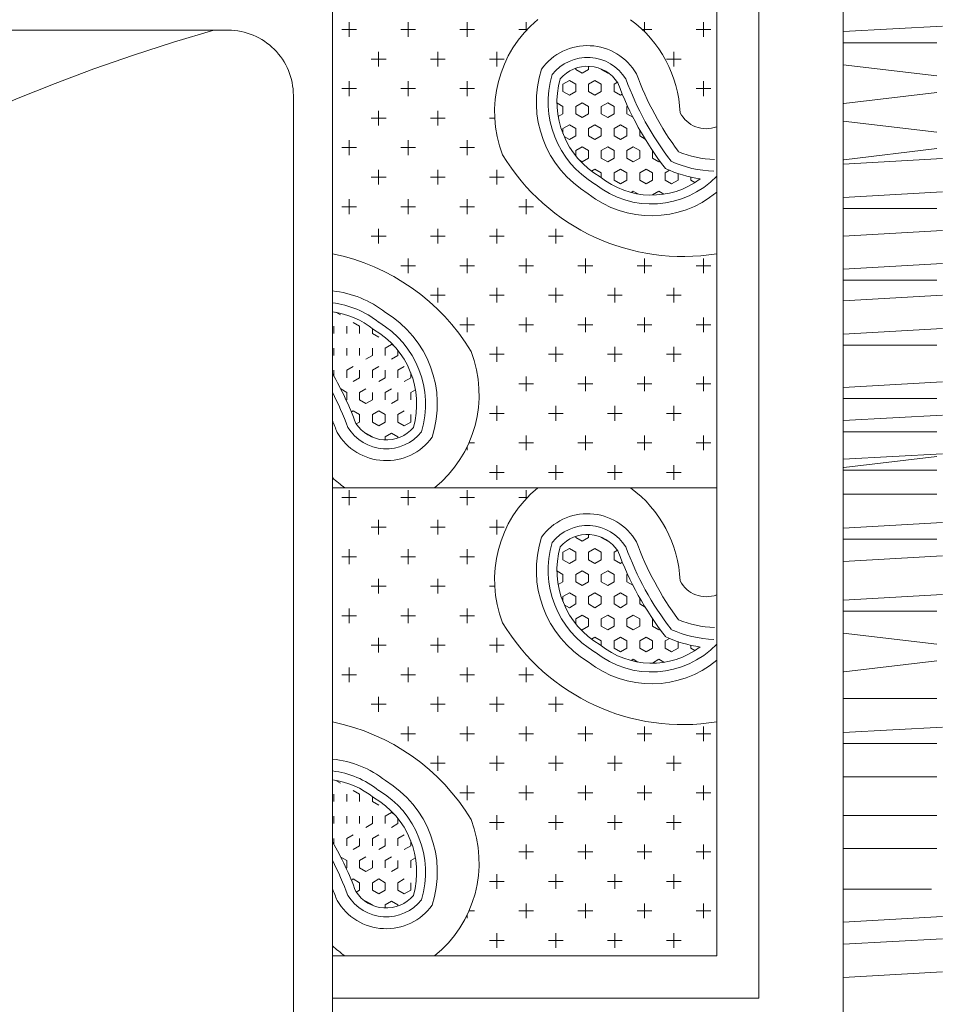
# Model space of a CAD drawing. Units: inches. Extents: x -638 to 186, y -762 to 59.
# Tile 9 of 31: x -117.58 to -100.41, y -492.33 to -474.18. Entities that reach past the tile are written whole.
import ezdxf

# ---------------------------------------------------------------- set-up
doc = ezdxf.new("R2010")
doc.units = ezdxf.units.IN
doc.layers.add('A-ANNO-DIMS', color=2, linetype='Continuous', lineweight=18)
doc.layers.add('furn', color=8, linetype='Continuous', lineweight=13)
doc.styles.get("Standard").update_dxf_attribs({"font": 'arial.ttf'})
doc.dimstyles.new('ISO-25', dxfattribs={"dimtxt": 4, "dimasz": 4, "dimexe": 1.25, "dimexo": 0.625, "dimtad": 0, "dimlunit": 4, "dimtxsty": 'Standard', "dimcen": 2.5, "dimclrt": 256, "dimadec": 0, "dimazin": 0, "dimtfac": 1, "dimtmove": 0, "dimatfit": 3, "dimfxl": 1, "dimfxlon": 1, "dimarcsym": 0})

# ---------------------------------------------------------------- blocks, each defined once
blk = doc.blocks.new('BED-DOUBLE-WITH-NIGHTSTANDS')
for p, q in [((57.828, 13.164), (57.828, 58.468)), ((22.077, 11.964), (56.628, 11.964)), ((20.158, 11.244), (58.548, 11.244)), ((39.99, 3.384), (39.99, 11.244)), ((40.767, 4.161), (40.767, 11.244)), ((42.588, 11.09), (42.524, 10.979)), ((42.932, 11.215), (42.819, 11.215)), ((43.34, 11.215), (43.204, 11.215)), ((43.748, 11.215), (43.612, 11.215)), ((44.002, 11.184), (43.952, 11.097)), ((45.948, 10.8), (45.948, 11.072)), ((47.036, 10.8), (47.036, 11.072)), ((48.125, 10.8), (48.125, 11.072)), ((49.213, 10.8), (49.213, 11.072)), ((49.395, 11.244), (49.395, 4.161)), ((51.216, 11.09), (51.151, 10.979)), ((51.56, 11.215), (51.447, 11.215)), ((51.968, 11.215), (51.832, 11.215)), ((52.376, 11.215), (52.24, 11.215)), ((52.63, 11.184), (52.58, 11.097)), ((54.576, 10.8), (54.576, 11.072)), ((55.664, 10.8), (55.664, 11.072)), ((56.752, 10.8), (56.752, 11.072)), ((57.841, 10.8), (57.841, 11.072)), ((42.164, 10.895), (42.184, 10.861)), ((42.381, 10.99), (42.388, 10.979)), ((42.524, 10.979), (42.388, 10.979)), ((42.932, 10.979), (42.796, 10.979)), ((42.932, 10.979), (43, 10.861)), ((43.34, 10.979), (43.204, 10.979)), ((43.748, 10.979), (43.612, 10.979)), ((45.812, 10.936), (46.084, 10.936)), ((46.9, 10.936), (47.172, 10.936)), ((47.989, 10.936), (48.261, 10.936)), ((49.077, 10.936), (49.349, 10.936)), ((50.792, 10.895), (50.811, 10.861)), ((51.009, 10.99), (51.015, 10.979)), ((51.151, 10.979), (51.015, 10.979)), ((51.56, 10.979), (51.424, 10.979)), ((51.56, 10.979), (51.628, 10.861)), ((51.968, 10.979), (51.832, 10.979)), ((52.376, 10.979), (52.24, 10.979)), ((54.44, 10.936), (54.712, 10.936)), ((55.528, 10.936), (55.8, 10.936)), ((56.616, 10.936), (56.888, 10.936)), ((57.705, 10.936), (57.977, 10.936)), ((41.943, 10.806), (41.98, 10.743)), ((42.116, 10.743), (41.98, 10.743)), ((42.184, 10.861), (42.116, 10.743)), ((42.388, 10.743), (42.32, 10.625)), ((42.524, 10.743), (42.388, 10.743)), ((42.524, 10.743), (42.592, 10.625)), ((42.728, 10.861), (42.796, 10.743)), ((42.932, 10.743), (42.796, 10.743)), ((43.34, 10.743), (43.204, 10.743)), ((43.748, 10.743), (43.612, 10.743)), ((43.816, 10.861), (43.748, 10.743)), ((50.571, 10.806), (50.607, 10.743)), ((50.743, 10.743), (50.607, 10.743)), ((50.811, 10.861), (50.743, 10.743)), ((51.015, 10.743), (50.947, 10.625)), ((51.151, 10.743), (51.015, 10.743)), ((51.151, 10.743), (51.219, 10.625)), ((51.355, 10.861), (51.424, 10.743)), ((51.56, 10.743), (51.424, 10.743)), ((51.968, 10.743), (51.832, 10.743)), ((52.376, 10.743), (52.24, 10.743)), ((52.444, 10.861), (52.376, 10.743)), ((41.776, 10.625), (41.708, 10.508)), ((41.77, 10.636), (41.776, 10.625)), ((42.32, 10.625), (42.388, 10.508)), ((43.136, 10.625), (43.204, 10.508)), ((45.404, 10.256), (45.404, 10.528)), ((46.492, 10.256), (46.492, 10.528)), ((47.581, 10.256), (47.581, 10.528)), ((48.669, 10.256), (48.669, 10.528)), ((50.403, 10.625), (50.335, 10.508)), ((50.397, 10.636), (50.403, 10.625)), ((50.947, 10.625), (51.015, 10.508)), ((51.764, 10.625), (51.832, 10.508)), ((54.032, 10.256), (54.032, 10.528)), ((55.12, 10.256), (55.12, 10.528)), ((56.208, 10.256), (56.208, 10.528)), ((57.297, 10.256), (57.297, 10.528)), ((41.708, 10.508), (41.699, 10.508)), ((41.98, 10.508), (41.912, 10.39)), ((41.912, 10.39), (41.98, 10.272)), ((42.116, 10.508), (41.98, 10.508)), ((42.116, 10.508), (42.184, 10.39)), ((42.184, 10.39), (42.116, 10.272)), ((42.524, 10.508), (42.388, 10.508)), ((42.728, 10.39), (42.796, 10.272)), ((42.932, 10.508), (42.796, 10.508)), ((42.932, 10.508), (43, 10.39)), ((43.34, 10.508), (43.204, 10.508)), ((43.612, 10.508), (43.544, 10.39)), ((43.703, 10.508), (43.612, 10.508)), ((45.268, 10.392), (45.54, 10.392)), ((46.356, 10.392), (46.628, 10.392)), ((47.445, 10.392), (47.717, 10.392)), ((48.533, 10.392), (48.805, 10.392)), ((50.335, 10.508), (50.327, 10.508)), ((50.607, 10.508), (50.539, 10.39)), ((50.539, 10.39), (50.607, 10.272)), ((50.743, 10.508), (50.607, 10.508)), ((50.743, 10.508), (50.811, 10.39)), ((50.811, 10.39), (50.743, 10.272)), ((51.151, 10.508), (51.015, 10.508)), ((51.355, 10.39), (51.424, 10.272)), ((51.56, 10.508), (51.424, 10.508)), ((51.56, 10.508), (51.628, 10.39)), ((51.968, 10.508), (51.832, 10.508)), ((52.24, 10.508), (52.172, 10.39)), ((52.33, 10.508), (52.24, 10.508)), ((53.896, 10.392), (54.168, 10.392)), ((54.984, 10.392), (55.256, 10.392)), ((56.072, 10.392), (56.344, 10.392)), ((57.161, 10.392), (57.433, 10.392)), ((41.708, 10.272), (41.649, 10.272)), ((41.708, 10.272), (41.776, 10.154)), ((42.116, 10.272), (41.98, 10.272)), ((42.524, 10.272), (42.388, 10.272)), ((42.524, 10.272), (42.592, 10.154)), ((42.932, 10.272), (42.796, 10.272)), ((43.34, 10.272), (43.204, 10.272)), ((43.34, 10.272), (43.408, 10.154)), ((50.335, 10.272), (50.277, 10.272)), ((50.335, 10.272), (50.403, 10.154)), ((50.743, 10.272), (50.607, 10.272)), ((51.151, 10.272), (51.015, 10.272)), ((51.151, 10.272), (51.219, 10.154)), ((51.56, 10.272), (51.424, 10.272)), ((51.968, 10.272), (51.832, 10.272)), ((51.968, 10.272), (52.036, 10.154)), ((41.708, 10.036), (41.685, 10.036)), ((41.776, 10.154), (41.708, 10.036)), ((41.98, 10.036), (41.912, 9.919)), ((42.116, 10.036), (41.98, 10.036)), ((42.116, 10.036), (42.184, 9.919)), ((42.32, 10.154), (42.388, 10.036)), ((42.524, 10.036), (42.388, 10.036)), ((42.932, 10.036), (42.796, 10.036)), ((42.932, 10.036), (43, 9.919)), ((43.136, 10.154), (43.204, 10.036)), ((43.297, 10.036), (43.204, 10.036)), ((43.408, 10.154), (43.381, 10.108)), ((44.86, 9.711), (44.86, 9.983)), ((45.948, 9.711), (45.948, 9.983)), ((47.036, 9.711), (47.036, 9.983)), ((48.125, 9.711), (48.125, 9.983)), ((49.213, 9.711), (49.213, 9.983)), ((50.335, 10.036), (50.313, 10.036)), ((50.403, 10.154), (50.335, 10.036)), ((50.607, 10.036), (50.539, 9.919)), ((50.743, 10.036), (50.607, 10.036)), ((50.743, 10.036), (50.811, 9.919)), ((50.947, 10.154), (51.015, 10.036)), ((51.151, 10.036), (51.015, 10.036)), ((51.56, 10.036), (51.424, 10.036)), ((51.56, 10.036), (51.628, 9.919)), ((51.764, 10.154), (51.832, 10.036)), ((51.925, 10.036), (51.832, 10.036)), ((52.036, 10.154), (52.009, 10.108)), ((53.487, 9.711), (53.487, 9.983)), ((54.576, 9.711), (54.576, 9.983)), ((55.664, 9.711), (55.664, 9.983)), ((56.752, 9.711), (56.752, 9.983)), ((57.841, 9.711), (57.841, 9.983)), ((41.912, 9.919), (41.98, 9.801)), ((42.116, 9.801), (41.98, 9.801)), ((42.524, 9.801), (42.388, 9.801)), ((42.524, 9.801), (42.574, 9.713)), ((42.728, 9.919), (42.796, 9.801)), ((42.888, 9.801), (42.796, 9.801)), ((44.724, 9.847), (44.996, 9.847)), ((45.812, 9.847), (46.084, 9.847)), ((46.9, 9.847), (47.172, 9.847)), ((47.989, 9.847), (48.261, 9.847)), ((49.077, 9.847), (49.349, 9.847)), ((50.539, 9.919), (50.607, 9.801)), ((50.743, 9.801), (50.607, 9.801)), ((51.151, 9.801), (51.015, 9.801)), ((51.151, 9.801), (51.202, 9.713)), ((51.355, 9.919), (51.424, 9.801)), ((51.516, 9.801), (51.424, 9.801)), ((53.351, 9.847), (53.623, 9.847)), ((54.44, 9.847), (54.712, 9.847)), ((55.528, 9.847), (55.8, 9.847)), ((56.616, 9.847), (56.888, 9.847)), ((57.705, 9.847), (57.977, 9.847)), ((44.316, 9.167), (44.316, 9.439)), ((45.404, 9.167), (45.404, 9.439)), ((46.492, 9.167), (46.492, 9.439)), ((47.581, 9.167), (47.581, 9.439)), ((48.669, 9.167), (48.669, 9.439)), ((52.943, 9.167), (52.943, 9.439)), ((54.032, 9.167), (54.032, 9.439)), ((55.12, 9.167), (55.12, 9.439)), ((56.208, 9.167), (56.208, 9.439)), ((57.297, 9.167), (57.297, 9.439)), ((44.18, 9.303), (44.452, 9.303)), ((45.268, 9.303), (45.54, 9.303)), ((46.356, 9.303), (46.628, 9.303)), ((47.445, 9.303), (47.717, 9.303)), ((48.533, 9.303), (48.805, 9.303)), ((52.807, 9.303), (53.079, 9.303)), ((53.896, 9.303), (54.168, 9.303)), ((54.984, 9.303), (55.256, 9.303)), ((56.072, 9.303), (56.344, 9.303)), ((57.161, 9.303), (57.433, 9.303)), ((43.771, 8.623), (43.771, 8.895)), ((44.86, 8.623), (44.86, 8.895)), ((45.948, 8.623), (45.948, 8.895)), ((47.036, 8.623), (47.036, 8.895)), ((48.125, 8.623), (48.125, 8.895)), ((49.213, 8.623), (49.213, 8.895)), ((52.399, 8.623), (52.399, 8.895)), ((53.487, 8.623), (53.487, 8.895)), ((54.576, 8.623), (54.576, 8.895)), ((55.664, 8.623), (55.664, 8.895)), ((56.752, 8.623), (56.752, 8.895)), ((57.841, 8.623), (57.841, 8.895)), ((41.459, 8.759), (41.528, 8.759)), ((41.595, 8.623), (41.595, 8.728)), ((43.635, 8.759), (43.907, 8.759)), ((44.724, 8.759), (44.996, 8.759)), ((45.812, 8.759), (46.084, 8.759)), ((46.9, 8.759), (47.172, 8.759)), ((47.989, 8.759), (48.261, 8.759)), ((49.077, 8.759), (49.349, 8.759)), ((50.086, 8.759), (50.155, 8.759)), ((50.222, 8.623), (50.222, 8.728)), ((52.263, 8.759), (52.535, 8.759)), ((53.351, 8.759), (53.623, 8.759)), ((54.44, 8.759), (54.712, 8.759)), ((55.528, 8.759), (55.8, 8.759)), ((56.616, 8.759), (56.888, 8.759)), ((57.705, 8.759), (57.977, 8.759)), ((41.051, 8.079), (41.051, 8.351)), ((42.139, 8.079), (42.139, 8.351)), ((43.227, 8.079), (43.227, 8.351)), ((44.316, 8.079), (44.316, 8.351)), ((45.404, 8.079), (45.404, 8.351)), ((46.492, 8.079), (46.492, 8.351)), ((47.581, 8.253), (47.581, 8.351)), ((48.669, 8.079), (48.669, 8.351)), ((49.678, 8.079), (49.678, 8.351)), ((50.767, 8.079), (50.767, 8.351)), ((51.855, 8.079), (51.855, 8.351)), ((52.943, 8.079), (52.943, 8.351)), ((54.032, 8.079), (54.032, 8.351)), ((55.12, 8.079), (55.12, 8.351)), ((56.208, 8.253), (56.208, 8.351)), ((57.297, 8.079), (57.297, 8.351)), ((40.914, 8.215), (41.187, 8.215)), ((42.003, 8.215), (42.275, 8.215)), ((43.091, 8.215), (43.363, 8.215)), ((44.18, 8.215), (44.452, 8.215)), ((45.268, 8.215), (45.54, 8.215)), ((46.356, 8.215), (46.628, 8.215)), ((48.533, 8.215), (48.805, 8.215)), ((49.542, 8.215), (49.814, 8.215)), ((50.63, 8.215), (50.903, 8.215)), ((51.719, 8.215), (51.991, 8.215)), ((52.807, 8.215), (53.079, 8.215)), ((53.896, 8.215), (54.168, 8.215)), ((54.984, 8.215), (55.256, 8.215)), ((57.161, 8.215), (57.433, 8.215)), ((41.595, 7.535), (41.595, 7.807)), ((42.683, 7.535), (42.683, 7.807)), ((43.771, 7.535), (43.771, 7.807)), ((44.86, 7.535), (44.86, 7.807)), ((45.948, 7.535), (45.948, 7.807)), ((49.213, 7.653), (49.213, 7.807)), ((50.222, 7.535), (50.222, 7.807)), ((51.311, 7.535), (51.311, 7.807)), ((52.399, 7.535), (52.399, 7.807)), ((53.487, 7.535), (53.487, 7.807)), ((54.576, 7.535), (54.576, 7.807)), ((57.841, 7.653), (57.841, 7.807)), ((41.459, 7.671), (41.731, 7.671)), ((42.547, 7.671), (42.819, 7.671)), ((43.635, 7.671), (43.907, 7.671)), ((44.724, 7.671), (44.996, 7.671)), ((45.812, 7.671), (46.084, 7.671)), ((49.195, 7.671), (49.349, 7.671)), ((50.086, 7.671), (50.358, 7.671)), ((51.175, 7.671), (51.447, 7.671)), ((52.263, 7.671), (52.535, 7.671)), ((53.351, 7.671), (53.623, 7.671)), ((54.44, 7.671), (54.712, 7.671)), ((57.822, 7.671), (57.977, 7.671)), ((41.051, 6.99), (41.051, 7.263)), ((42.139, 6.99), (42.139, 7.263)), ((43.227, 6.99), (43.227, 7.263)), ((44.316, 6.99), (44.316, 7.263)), ((45.404, 6.99), (45.404, 7.263)), ((49.678, 6.99), (49.678, 7.263)), ((50.767, 6.99), (50.767, 7.263)), ((51.855, 6.99), (51.855, 7.263)), ((52.943, 6.99), (52.943, 7.263)), ((54.032, 6.99), (54.032, 7.263)), ((40.914, 7.127), (41.187, 7.127)), ((42.003, 7.127), (42.275, 7.127)), ((43.091, 7.127), (43.363, 7.127)), ((44.18, 7.127), (44.452, 7.127)), ((45.268, 7.127), (45.54, 7.127)), ((47.661, 6.995), (47.611, 7.082)), ((47.797, 6.995), (47.861, 7.105)), ((49.542, 7.127), (49.814, 7.127)), ((50.63, 7.127), (50.903, 7.127)), ((51.719, 7.127), (51.991, 7.127)), ((52.807, 7.127), (53.079, 7.127)), ((53.896, 7.127), (54.168, 7.127)), ((56.289, 6.995), (56.238, 7.082)), ((56.425, 6.995), (56.488, 7.105)), ((47.185, 6.877), (47.239, 6.971)), ((47.297, 6.995), (47.389, 6.995)), ((47.457, 6.877), (47.389, 6.995)), ((47.661, 6.995), (47.797, 6.995)), ((48.001, 6.877), (48.069, 6.995)), ((48.069, 6.995), (48.205, 6.995)), ((48.273, 6.877), (48.205, 6.995)), ((55.813, 6.877), (55.867, 6.971)), ((55.924, 6.995), (56.017, 6.995)), ((56.085, 6.877), (56.017, 6.995)), ((56.289, 6.995), (56.425, 6.995)), ((56.629, 6.877), (56.697, 6.995)), ((56.697, 6.995), (56.833, 6.995)), ((56.901, 6.877), (56.833, 6.995)), ((41.595, 6.446), (41.595, 6.718)), ((42.683, 6.446), (42.683, 6.718)), ((43.771, 6.446), (43.771, 6.718)), ((44.86, 6.446), (44.86, 6.718)), ((46.888, 6.76), (46.981, 6.76)), ((47.049, 6.642), (46.981, 6.76)), ((47.253, 6.76), (47.185, 6.877)), ((47.253, 6.76), (47.389, 6.76)), ((47.389, 6.76), (47.457, 6.877)), ((47.593, 6.642), (47.661, 6.76)), ((47.661, 6.76), (47.797, 6.76)), ((47.865, 6.642), (47.797, 6.76)), ((48.069, 6.76), (48.001, 6.877)), ((48.069, 6.76), (48.205, 6.76)), ((48.205, 6.76), (48.273, 6.877)), ((48.409, 6.642), (48.477, 6.76)), ((48.477, 6.76), (48.5, 6.76)), ((50.222, 6.446), (50.222, 6.718)), ((51.311, 6.446), (51.311, 6.718)), ((52.399, 6.446), (52.399, 6.718)), ((53.487, 6.446), (53.487, 6.718)), ((55.515, 6.76), (55.609, 6.76)), ((55.677, 6.642), (55.609, 6.76)), ((55.881, 6.76), (55.813, 6.877)), ((55.881, 6.76), (56.017, 6.76)), ((56.017, 6.76), (56.085, 6.877)), ((56.221, 6.642), (56.289, 6.76)), ((56.289, 6.76), (56.425, 6.76)), ((56.493, 6.642), (56.425, 6.76)), ((56.697, 6.76), (56.629, 6.877)), ((56.697, 6.76), (56.833, 6.76)), ((56.833, 6.76), (56.901, 6.877)), ((57.037, 6.642), (57.105, 6.76)), ((57.105, 6.76), (57.128, 6.76)), ((41.459, 6.582), (41.731, 6.582)), ((42.547, 6.582), (42.819, 6.582)), ((43.635, 6.582), (43.907, 6.582)), ((44.724, 6.582), (44.996, 6.582)), ((46.777, 6.642), (46.803, 6.688)), ((46.845, 6.524), (46.777, 6.642)), ((46.981, 6.524), (47.049, 6.642)), ((47.661, 6.524), (47.593, 6.642)), ((47.797, 6.524), (47.865, 6.642)), ((48.477, 6.524), (48.409, 6.642)), ((50.086, 6.582), (50.358, 6.582)), ((51.175, 6.582), (51.447, 6.582)), ((52.263, 6.582), (52.535, 6.582)), ((53.351, 6.582), (53.623, 6.582)), ((55.405, 6.642), (55.431, 6.688)), ((55.473, 6.524), (55.405, 6.642)), ((55.609, 6.524), (55.677, 6.642)), ((56.289, 6.524), (56.221, 6.642)), ((56.425, 6.524), (56.493, 6.642)), ((57.105, 6.524), (57.037, 6.642)), ((46.573, 6.288), (46.641, 6.406)), ((46.641, 6.406), (46.605, 6.469)), ((46.845, 6.524), (46.981, 6.524)), ((47.185, 6.406), (47.253, 6.524)), ((47.253, 6.288), (47.185, 6.406)), ((47.253, 6.524), (47.389, 6.524)), ((47.457, 6.406), (47.389, 6.524)), ((47.389, 6.288), (47.457, 6.406)), ((47.661, 6.524), (47.797, 6.524)), ((48.001, 6.406), (48.069, 6.524)), ((48.069, 6.288), (48.001, 6.406)), ((48.069, 6.524), (48.205, 6.524)), ((48.273, 6.406), (48.205, 6.524)), ((48.205, 6.288), (48.273, 6.406)), ((48.477, 6.524), (48.536, 6.524)), ((55.201, 6.288), (55.269, 6.406)), ((55.269, 6.406), (55.232, 6.469)), ((55.473, 6.524), (55.609, 6.524)), ((55.813, 6.406), (55.881, 6.524)), ((55.881, 6.288), (55.813, 6.406)), ((55.881, 6.524), (56.017, 6.524)), ((56.085, 6.406), (56.017, 6.524)), ((56.017, 6.288), (56.085, 6.406)), ((56.289, 6.524), (56.425, 6.524)), ((56.629, 6.406), (56.697, 6.524)), ((56.697, 6.288), (56.629, 6.406)), ((56.697, 6.524), (56.833, 6.524)), ((56.901, 6.406), (56.833, 6.524)), ((56.833, 6.288), (56.901, 6.406)), ((57.105, 6.524), (57.164, 6.524)), ((41.051, 5.902), (41.051, 6.174)), ((42.139, 5.902), (42.139, 6.174)), ((43.227, 5.902), (43.227, 6.174)), ((44.316, 5.902), (44.316, 6.174)), ((46.482, 6.288), (46.573, 6.288)), ((46.777, 6.17), (46.845, 6.288)), ((46.845, 6.053), (46.777, 6.17)), ((46.845, 6.288), (46.981, 6.288)), ((47.049, 6.17), (46.981, 6.288)), ((46.981, 6.053), (47.049, 6.17)), ((47.253, 6.288), (47.389, 6.288)), ((47.593, 6.17), (47.661, 6.288)), ((47.661, 6.053), (47.593, 6.17)), ((47.661, 6.288), (47.797, 6.288)), ((47.865, 6.17), (47.797, 6.288)), ((47.797, 6.053), (47.865, 6.17)), ((48.069, 6.288), (48.205, 6.288)), ((48.409, 6.17), (48.477, 6.288)), ((48.415, 6.16), (48.409, 6.17)), ((48.477, 6.288), (48.486, 6.288)), ((49.678, 5.902), (49.678, 6.174)), ((50.767, 5.902), (50.767, 6.174)), ((51.855, 5.902), (51.855, 6.174)), ((52.943, 5.902), (52.943, 6.174)), ((55.11, 6.288), (55.201, 6.288)), ((55.405, 6.17), (55.473, 6.288)), ((55.473, 6.053), (55.405, 6.17)), ((55.473, 6.288), (55.609, 6.288)), ((55.677, 6.17), (55.609, 6.288)), ((55.609, 6.053), (55.677, 6.17)), ((55.881, 6.288), (56.017, 6.288)), ((56.221, 6.17), (56.289, 6.288)), ((56.289, 6.053), (56.221, 6.17)), ((56.289, 6.288), (56.425, 6.288)), ((56.493, 6.17), (56.425, 6.288)), ((56.425, 6.053), (56.493, 6.17)), ((56.697, 6.288), (56.833, 6.288)), ((57.037, 6.17), (57.105, 6.288)), ((57.043, 6.16), (57.037, 6.17)), ((57.105, 6.288), (57.113, 6.288)), ((40.914, 6.038), (41.187, 6.038)), ((42.003, 6.038), (42.275, 6.038)), ((43.091, 6.038), (43.363, 6.038)), ((44.18, 6.038), (44.452, 6.038)), ((46.369, 5.935), (46.437, 6.053)), ((46.437, 6.053), (46.573, 6.053)), ((46.641, 5.935), (46.573, 6.053)), ((46.845, 6.053), (46.981, 6.053)), ((47.185, 5.935), (47.253, 6.053)), ((47.253, 6.053), (47.389, 6.053)), ((47.457, 5.935), (47.389, 6.053)), ((47.661, 6.053), (47.797, 6.053)), ((48.001, 5.935), (48.069, 6.053)), ((48.069, 6.053), (48.205, 6.053)), ((48.242, 5.99), (48.205, 6.053)), ((49.542, 6.038), (49.814, 6.038)), ((50.63, 6.038), (50.903, 6.038)), ((51.719, 6.038), (51.991, 6.038)), ((52.807, 6.038), (53.079, 6.038)), ((54.996, 5.935), (55.064, 6.053)), ((55.064, 6.053), (55.201, 6.053)), ((55.269, 5.935), (55.201, 6.053)), ((55.473, 6.053), (55.609, 6.053)), ((55.813, 5.935), (55.881, 6.053)), ((55.881, 6.053), (56.017, 6.053)), ((56.085, 5.935), (56.017, 6.053)), ((56.289, 6.053), (56.425, 6.053)), ((56.629, 5.935), (56.697, 6.053)), ((56.697, 6.053), (56.833, 6.053)), ((56.869, 5.99), (56.833, 6.053)), ((46.437, 5.817), (46.369, 5.935)), ((46.437, 5.817), (46.573, 5.817)), ((46.573, 5.817), (46.641, 5.935)), ((46.777, 5.699), (46.845, 5.817)), ((46.845, 5.817), (46.981, 5.817)), ((47.049, 5.699), (46.981, 5.817)), ((47.253, 5.817), (47.185, 5.935)), ((47.253, 5.817), (47.389, 5.817)), ((47.389, 5.817), (47.457, 5.935)), ((47.597, 5.706), (47.661, 5.817)), ((47.661, 5.817), (47.797, 5.817)), ((47.804, 5.806), (47.797, 5.817)), ((48.021, 5.901), (48.001, 5.935)), ((55.064, 5.817), (54.996, 5.935)), ((55.064, 5.817), (55.201, 5.817)), ((55.201, 5.817), (55.269, 5.935)), ((55.405, 5.699), (55.473, 5.817)), ((55.473, 5.817), (55.609, 5.817)), ((55.677, 5.699), (55.609, 5.817)), ((55.881, 5.817), (55.813, 5.935)), ((55.881, 5.817), (56.017, 5.817)), ((56.017, 5.817), (56.085, 5.935)), ((56.225, 5.706), (56.289, 5.817)), ((56.289, 5.817), (56.425, 5.817)), ((56.431, 5.806), (56.425, 5.817)), ((56.649, 5.901), (56.629, 5.935)), ((41.595, 5.358), (41.595, 5.63)), ((42.683, 5.358), (42.683, 5.63)), ((43.771, 5.358), (43.771, 5.63)), ((44.86, 5.358), (44.86, 5.63)), ((46.183, 5.612), (46.233, 5.699)), ((46.233, 5.699), (46.21, 5.739)), ((46.845, 5.581), (46.777, 5.699)), ((46.981, 5.581), (47.049, 5.699)), ((50.222, 5.358), (50.222, 5.63)), ((51.311, 5.358), (51.311, 5.63)), ((52.399, 5.358), (52.399, 5.63)), ((53.487, 5.358), (53.487, 5.63)), ((54.81, 5.612), (54.86, 5.699)), ((54.86, 5.699), (54.837, 5.739)), ((55.473, 5.581), (55.405, 5.699)), ((55.609, 5.581), (55.677, 5.699)), ((41.459, 5.494), (41.731, 5.494)), ((42.547, 5.494), (42.819, 5.494)), ((43.635, 5.494), (43.907, 5.494)), ((44.724, 5.494), (44.996, 5.494)), ((46.369, 5.464), (46.437, 5.581)), ((46.437, 5.346), (46.369, 5.464)), ((46.437, 5.581), (46.573, 5.581)), ((46.641, 5.464), (46.573, 5.581)), ((46.573, 5.346), (46.641, 5.464)), ((46.845, 5.581), (46.981, 5.581)), ((47.195, 5.481), (47.253, 5.581)), ((47.253, 5.581), (47.365, 5.581)), ((50.086, 5.494), (50.358, 5.494)), ((51.175, 5.494), (51.447, 5.494)), ((52.263, 5.494), (52.535, 5.494)), ((53.351, 5.494), (53.623, 5.494)), ((54.996, 5.464), (55.064, 5.581)), ((55.064, 5.346), (54.996, 5.464)), ((55.064, 5.581), (55.201, 5.581)), ((55.269, 5.464), (55.201, 5.581)), ((55.201, 5.346), (55.269, 5.464)), ((55.473, 5.581), (55.609, 5.581)), ((55.823, 5.481), (55.881, 5.581)), ((55.881, 5.581), (55.993, 5.581)), ((57.803, 5.494), (57.977, 5.494)), ((57.841, 5.358), (57.841, 5.533)), ((46.162, 5.346), (46.165, 5.346)), ((46.233, 5.228), (46.165, 5.346)), ((46.437, 5.346), (46.573, 5.346)), ((46.777, 5.228), (46.845, 5.346)), ((46.845, 5.346), (46.981, 5.346)), ((46.982, 5.344), (46.981, 5.346)), ((54.789, 5.346), (54.792, 5.346)), ((54.86, 5.228), (54.792, 5.346)), ((55.064, 5.346), (55.201, 5.346)), ((55.405, 5.228), (55.473, 5.346)), ((55.473, 5.346), (55.609, 5.346)), ((55.609, 5.344), (55.609, 5.346)), ((41.051, 4.814), (41.051, 5.086)), ((42.139, 4.814), (42.139, 5.086)), ((43.227, 4.814), (43.227, 5.086)), ((44.316, 4.814), (44.316, 5.086)), ((46.179, 5.135), (46.233, 5.228)), ((46.369, 4.992), (46.437, 5.11)), ((46.437, 5.11), (46.573, 5.11)), ((46.619, 5.03), (46.573, 5.11)), ((46.788, 5.209), (46.777, 5.228)), ((49.678, 4.814), (49.678, 5.086)), ((50.767, 4.814), (50.767, 5.086)), ((51.855, 4.814), (51.855, 5.086)), ((52.943, 4.814), (52.943, 5.086)), ((54.807, 5.135), (54.86, 5.228)), ((54.996, 4.992), (55.064, 5.11)), ((55.064, 5.11), (55.201, 5.11)), ((55.247, 5.03), (55.201, 5.11)), ((55.416, 5.209), (55.405, 5.228)), ((57.297, 4.814), (57.297, 5.086)), ((40.914, 4.95), (41.187, 4.95)), ((42.003, 4.95), (42.275, 4.95)), ((43.091, 4.95), (43.363, 4.95)), ((44.18, 4.95), (44.452, 4.95)), ((46.437, 4.874), (46.369, 4.992)), ((49.542, 4.95), (49.814, 4.95)), ((50.63, 4.95), (50.903, 4.95)), ((51.719, 4.95), (51.991, 4.95)), ((52.807, 4.95), (53.079, 4.95)), ((55.064, 4.874), (54.996, 4.992)), ((57.161, 4.95), (57.433, 4.95)), ((46.437, 4.874), (46.559, 4.874)), ((55.064, 4.874), (55.187, 4.874)), ((41.595, 4.27), (41.595, 4.542)), ((42.683, 4.27), (42.683, 4.542)), ((43.771, 4.27), (43.771, 4.542)), ((44.86, 4.27), (44.86, 4.542)), ((46.393, 4.563), (46.437, 4.639)), ((46.437, 4.639), (46.493, 4.639)), ((50.222, 4.27), (50.222, 4.542)), ((51.311, 4.27), (51.311, 4.542)), ((52.399, 4.27), (52.399, 4.542)), ((53.487, 4.27), (53.487, 4.542)), ((55.021, 4.563), (55.064, 4.639)), ((55.064, 4.639), (55.12, 4.639)), ((56.752, 4.27), (56.752, 4.542)), ((57.841, 4.27), (57.841, 4.542)), ((41.459, 4.406), (41.731, 4.406)), ((42.547, 4.406), (42.819, 4.406)), ((43.635, 4.406), (43.907, 4.406)), ((44.724, 4.406), (44.996, 4.406)), ((50.086, 4.406), (50.358, 4.406)), ((51.175, 4.406), (51.447, 4.406)), ((52.263, 4.406), (52.535, 4.406)), ((53.351, 4.406), (53.623, 4.406)), ((56.616, 4.406), (56.888, 4.406)), ((57.705, 4.406), (57.977, 4.406)), ((66.65, 4.161), (40.767, 4.161)), ((67.427, 3.384), (39.99, 3.384)), ((68.982, 1.829), (38.435, 1.829)), ((40.369, 1.829), (40.471, 0)), ((40.98, 1.829), (41.082, 0)), ((41.388, 1.829), (41.49, 0)), ((41.999, 1.829), (41.999, 0.203)), ((42.744, 1.829), (42.744, 0.102)), ((43.355, 1.829), (43.355, 0.102)), ((44.068, 1.829), (44.068, 0.102)), ((44.679, 1.829), (44.679, 0.102)), ((44.882, 1.829), (44.984, 0)), ((45.511, 1.815), (45.511, 0.105)), ((46.002, 1.815), (46.206, 0.102)), ((46.715, 1.829), (46.512, 0.102)), ((47.122, 1.829), (47.122, 0.102)), ((47.326, 1.829), (47.428, 0)), ((48.039, 1.829), (48.141, 0)), ((48.446, 1.829), (48.446, 0.102)), ((48.65, 1.829), (48.752, 0)), ((49.279, 1.815), (49.279, 0.105)), ((49.717, 1.829), (49.717, 0.102)), ((49.77, 1.815), (49.973, 0.102)), ((49.92, 1.829), (50.022, 0)), ((50.429, 1.829), (50.429, 0.102)), ((50.633, 1.829), (50.735, 0)), ((51.04, 1.829), (51.04, 0.102)), ((51.244, 1.829), (51.346, 0)), ((52.025, 1.829), (52.025, 0.102)), ((52.229, 1.829), (52.331, 0)), ((52.84, 1.829), (52.942, 0)), ((53.221, 1.829), (53.221, 0.102)), ((53.424, 1.829), (53.526, 0)), ((54.035, 1.829), (54.137, 0)), ((54.544, 1.829), (54.544, 0.102)), ((54.748, 1.829), (54.85, 0)), ((55.359, 1.829), (55.461, 0)), ((55.442, 1.815), (55.646, 0.102)), ((56.155, 1.829), (55.951, 0.102)), ((56.479, 1.815), (56.683, 0.102)), ((57.192, 1.829), (56.988, 0.102)), ((57.599, 1.829), (57.599, 0.102)), ((57.803, 1.829), (57.905, 0))]:
    blk.add_line(p, q)
for centre, radius, start, end in [((27.358, 4.824), 31.662, 15.7708, 101.8099), ((56.628, 13.164), 1.2, 270, 360), ((42.601, 9.717), 2.246, 137.1431, 144.7393), ((42.315, 10.253), 1.047, 120.344, 234.0192), ((39.887, 16.395), 5.571, 289.9219, 292.4118), ((39.887, 16.395), 5.789, 290.1318, 297.1635), ((39.887, 16.395), 5.952, 290.2997, 300.0824), ((41.275, 12.01), 3.88, 301.1125, 348.6139), ((42.526, 11.434), 1.497, 320.6541, 352.729), ((42.526, 11.434), 1.66, 321.1107, 353.4472), ((42.526, 11.434), 1.878, 321.5973, 354.2094), ((51.228, 9.717), 2.246, 137.1431, 144.7393), ((50.942, 10.253), 1.047, 120.344, 234.0192), ((48.515, 16.395), 5.571, 289.9219, 292.4118), ((48.515, 16.395), 5.789, 290.1318, 297.1635), ((48.515, 16.395), 5.952, 290.2997, 300.0824), ((49.903, 12.01), 3.88, 301.1125, 348.6139), ((51.154, 11.434), 1.497, 320.6541, 352.729), ((51.154, 11.434), 1.66, 321.1107, 353.4472), ((51.154, 11.434), 1.878, 321.5973, 354.2094), ((42.315, 10.253), 0.829, 121.6232, 231.6957), ((50.942, 10.253), 0.829, 121.6232, 231.6957), ((42.315, 10.253), 0.666, 122.9498, 229.099), ((50.942, 10.253), 0.666, 122.9498, 229.099), ((42.307, 11.282), 1.754, 253.2189, 329.4808), ((42.307, 11.282), 1.591, 254.3738, 329.9117), ((50.935, 11.282), 1.754, 253.2189, 329.4808), ((50.935, 11.282), 1.591, 254.3738, 329.9117), ((42.307, 11.282), 1.972, 252.055, 329.019), ((50.935, 11.282), 1.972, 252.055, 329.019), ((42.485, 10.742), 2.202, 218.7027, 291.1583), ((51.113, 10.742), 2.202, 218.7027, 291.1583), ((47.7, 6.054), 2.202, 39.6653, 111.1583), ((56.328, 6.054), 2.202, 39.6653, 111.1583), ((48.91, 4.786), 3.88, 121.1125, 189.2666), ((57.538, 4.786), 3.88, 121.1125, 189.2666), ((47.878, 5.514), 1.972, 72.055, 149.019), ((56.505, 5.514), 1.972, 72.055, 149.019), ((47.878, 5.514), 1.754, 73.2189, 149.4808), ((47.87, 6.543), 1.047, 300.344, 54.0192), ((56.505, 5.514), 1.754, 73.2189, 149.4808), ((56.498, 6.543), 1.047, 300.344, 54.0192), ((47.878, 5.514), 1.591, 74.3738, 149.9117), ((47.87, 6.543), 0.829, 301.6232, 51.6957), ((56.505, 5.514), 1.591, 74.3738, 149.9117), ((56.498, 6.543), 0.829, 301.6232, 51.6957), ((47.87, 6.543), 0.666, 302.9498, 49.099), ((56.498, 6.543), 0.666, 302.9498, 49.099), ((47.659, 5.362), 1.878, 141.5973, 219.7611), ((47.659, 5.362), 1.66, 141.1107, 226.3387), ((56.286, 5.362), 1.878, 141.5973, 219.7611), ((56.286, 5.362), 1.66, 141.1107, 226.3387), ((47.659, 5.362), 1.497, 140.6541, 216.833), ((56.286, 5.362), 1.497, 140.6541, 216.833), ((50.298, 0.401), 5.952, 110.2997, 127.7385), ((50.298, 0.401), 5.789, 110.1318, 127.346), ((58.925, 0.401), 5.952, 110.2997, 127.7385), ((58.925, 0.401), 5.789, 110.1318, 127.346), ((50.298, 0.401), 5.571, 109.9219, 126.7677), ((47.584, 7.079), 2.246, 272.4675, 323.7193), ((58.925, 0.401), 5.571, 109.9219, 126.7677), ((56.212, 7.079), 2.246, 272.4675, 323.7193), ((48.704, 4.14), 2.268, 154.7059, 171.7535), ((57.332, 4.14), 2.268, 154.7059, 171.7535), ((48.704, 4.14), 2.104, 155.7609, 178.0373), ((57.332, 4.14), 2.104, 155.7609, 178.0373), ((48.704, 4.14), 1.887, 157.4091, 178.0373), ((47.926, 4.355), 0.54, 117.0088, 201.0409), ((57.332, 4.14), 1.887, 157.4091, 178.0373), ((56.554, 4.355), 0.54, 117.0088, 201.0409)]:
    blk.add_arc(centre, radius, start, end)
blk = doc.blocks.new('*D38')
at = {"layer": 'A-ANNO-DIMS', "color": 0, "lineweight": -2, "transparency": 16777216}
for p, q in [((182.663, -280.533), (184.913, -280.533)), ((183.663, -284.533), (183.663, -371.726)), ((183.663, -473.533), (183.663, -386.34)), ((182.663, -477.533), (184.913, -477.533))]:
    blk.add_line(p, q, dxfattribs=at)
at = {"layer": 'A-ANNO-DIMS', "color": 0, "lineweight": 30, "transparency": 16777216}
for points in [[(182.997, -284.533), (184.33, -284.533), (183.663, -280.533)], [(182.997, -473.533), (184.33, -473.533), (183.663, -477.533)]]:
    blk.add_solid(points, dxfattribs=at)
at = {"layer": 'Defpoints', "color": 0, "lineweight": 30, "transparency": 16777216}
for p in [(-404.526, -280.533), (-404.526, -477.533), (183.663, -477.533)]:
    blk.add_point(p, dxfattribs=at)
at = {"layer": 'A-ANNO-DIMS', "transparency": 16777216, "insert": (183.663, -379.033), "char_height": 4, "attachment_point": 5, "rotation": 90}
blk.add_mtext('16\'-5"', dxfattribs=at)

msp = doc.modelspace()

# ---------------------------------------------------------------- block references
at = {"layer": 'furn', "rotation": 90.00000000000017}
msp.add_blockref('BED-DOUBLE-WITH-NIGHTSTANDS', (-100.575, -532.203), dxfattribs=at)

# ---------------------------------------------------------------- dimensions: what is measured, and where the dimension line sits
at = {"layer": 'A-ANNO-DIMS'}
dim = msp.add_linear_dim(base=(183.663, -477.533), p1=(-404.526, -280.533), p2=(-404.526, -477.533), angle=90, dimstyle='ISO-25', override={"dimdec": 1, "dimlfac": 1, "dimrnd": 0, "dimzin": 1, "dimdsep": 46, "dimlunit": 4, "dimfrac": 2}, dxfattribs=at)
dim.commit()
dim.dimension.update_dxf_attribs({"geometry": '*D38', "text_midpoint": (183.663, -379.033)})

doc.saveas('drawing.dxf')
